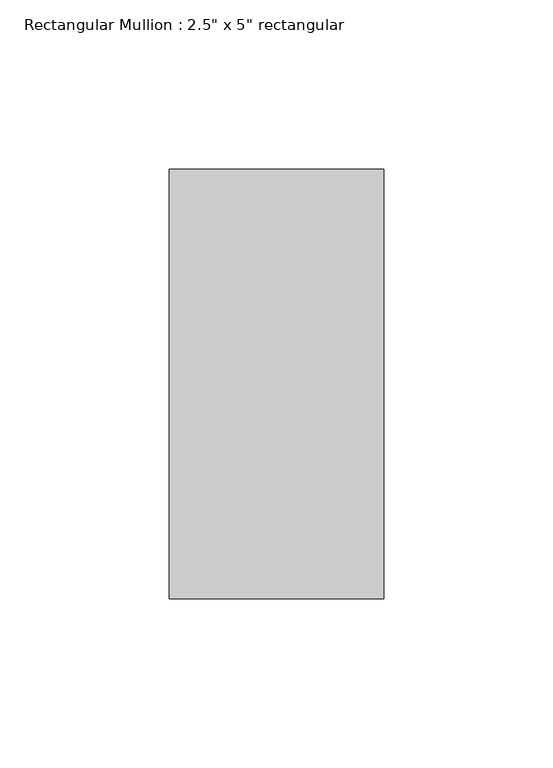
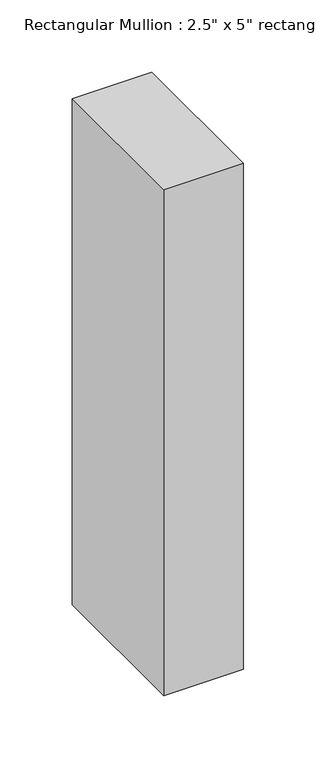
"""IFC4 building model written with IfcOpenShell, lengths in millimetres: member geometry."""

from ifc_helpers import new_model, si_unit, frame, origin, place, context, project, spatial, polyline, outline, extrude, source, transform, mapped, element, save


def member_39486dda(model_context):
    return source(origin(), model_context, "Body", "SweptSolid", [
        extrude(outline(polyline([(0.0, 63.5), (0.0, -63.5), (-63.5, -63.5), (-63.5, 63.5), (0.0, 63.5)])), frame((0.0, 0.0, -427.5666667), z_axis=(0.0, 0.0, 1.0), x_axis=(1.0, 0.0, 0.0)), (0.0, 0.0, 1.0), 427.5666667),
    ])


if __name__ == "__main__":
    model = new_model("IFC4")
    model_context = context("Model", 3, world=origin())
    ifc_project = project(units=[si_unit("LENGTHUNIT", "METRE", prefix="MILLI")], contexts=[model_context])
    site = spatial("IfcSite", under=ifc_project)
    building = spatial("IfcBuilding", under=site)
    placement = place(None, origin())
    member_shape = member_39486dda(model_context)
    element("IfcMember", 1, ObjectType="Rectangular Mullion : 2.5\" x 5\" rectangular", at=placement, inside=building, context=model_context, shape_type="MappedRepresentation", body=[
        mapped(member_shape, transform((0.0, 0.0, 0.0), x_axis=(1.0, 0.0, 0.0), y_axis=(0.0, 1.0, 0.0), z_axis=(0.0, 0.0, 1.0))),
    ])
    save(model, "model.ifc")

# Revit data of these elements
# Type "Rectangular Mullion : 2.5\" x 5\" rectangular"
#   built-in parameter 1007304 = 0.416667 (stored number, unit not read)
#   built-in parameter 1007301 = 0.104167 (stored number, unit not read)
#   built-in parameter 1007300 = 0.104167 (stored number, unit not read)
